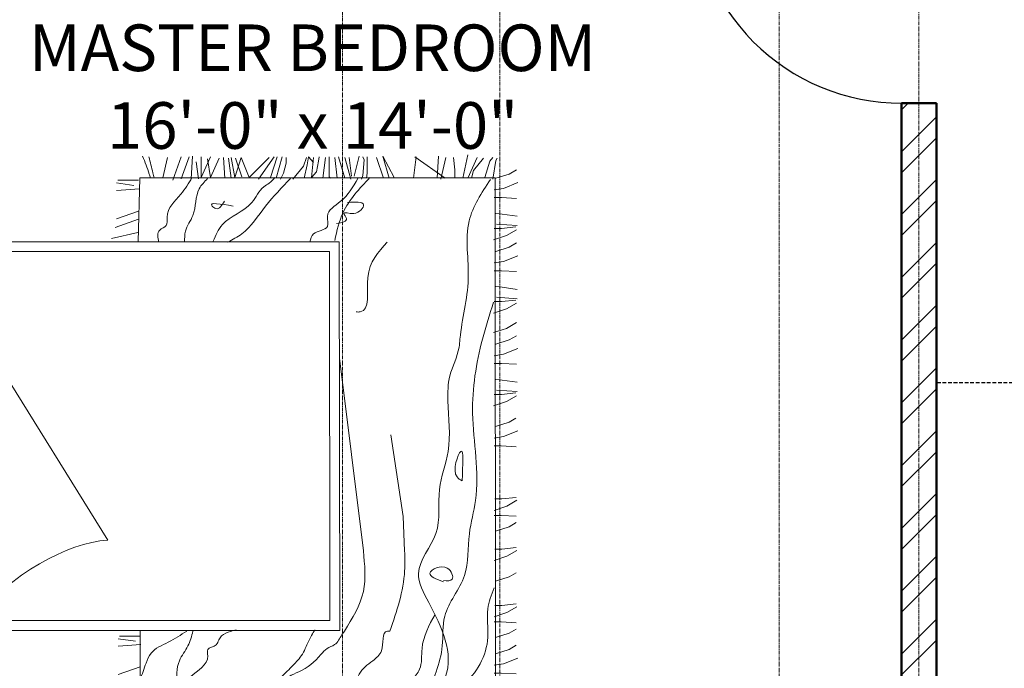
# Model space of a CAD drawing. Units: inches. Extents: x 261 to 2725, y 291 to 1454.
# Tile 5 of 35: x 519 to 688, y 549 to 661. Entities that reach past the tile are written whole.
import ezdxf

# ---------------------------------------------------------------- set-up
doc = ezdxf.new("R2010")
doc.units = ezdxf.units.IN
doc.linetypes.add('CENTER', pattern=[2, 1.25, -0.25, 0.25, -0.25])
doc.linetypes.add('DASHED', pattern=[19.05, 12.7, -6.35])
for name, color, linetype, lineweight in [('A-ANNO-DIMS', 136, 'Continuous', 18), ('A-AREA-IDEN', 18, 'Continuous', 18), ('A-DOOR', 160, 'Continuous', 25), ('A-FURN', 30, 'Continuous', 18), ('A-GRID', 251, 'CENTER', 13), ('A-WALL', 222, 'Continuous', 50), ('A-WALL-OVHD', 222, 'DASHED', 25), ('A-WALL-PATT', 243, 'Continuous', 13)]:
    doc.layers.add(name, color=color, linetype=linetype, lineweight=lineweight)
doc.styles.get("Standard").update_dxf_attribs({"font": 'arial.ttf'})
doc.dimstyles.new('ISO-25', dxfattribs={"dimtxt": 12, "dimasz": 6, "dimexe": 1.25, "dimexo": 0.625, "dimtad": 1, "dimdec": 0, "dimlunit": 3, "dimtxsty": 'Standard', "dimblk": 'ARCHTICK', "dimcen": 2.5, "dimadec": 0, "dimazin": 0, "dimtfac": 1, "dimtdec": 0, "dimtmove": 0, "dimatfit": 3, "dimfxl": 1, "dimfxlon": 1, "dimarcsym": 0})

# ---------------------------------------------------------------- blocks, each defined once
blk = doc.blocks.new('*U5')
for p, q in [((0, 0), (0, -4)), ((-36, 0), (-36, -4))]:
    blk.add_line(p, q)
blk.add_lwpolyline([(0, 0), (0, 36), (-1.75, 36), (-1.75, 0)], close=True)
blk.add_arc((0, 0), 36, 90, 180)
blk = doc.blocks.new('A$C2B723114')
for p, q in [((0, 2.9047), (2.8274, 2.9047)), ((0, 2.8487), (0, 2.9047)), ((2.8274, 2.9047), (2.8274, 2.8487)), ((2.8274, 2.8487), (0, 2.8487)), ((0.1012, 2.4649), (0.1012, 2.849)), ((0.1396, 2.5033), (0.1396, 2.849)), ((0.4243, 2.8697), (0.4243, 2.4855)), ((0.6794, 0.7051), (0.6794, 2.8509)), ((0.7187, 0.7435), (0.7187, 2.8509)), ((2.1776, 2.8509), (2.1776, 0.7454)), ((2.216, 2.8509), (2.216, 0.707)), ((2.4742, 2.8697), (2.4742, 2.4855)), ((2.6798, 2.5052), (2.6798, 2.8509)), ((2.7182, 2.4668), (2.7182, 2.8509)), ((0.6087, 2.6776), (0.295, 2.6776)), ((2.6586, 2.6776), (2.2821, 2.6776)), ((1.3789, 2.4999), (1.3598, 2.5761)), ((2.0593, 2.4999), (2.0402, 2.5761)), ((0.6766, 2.5033), (0.1396, 2.5033)), ((1.3858, 2.4723), (1.3789, 2.4999)), ((2.0662, 2.4723), (2.0593, 2.4999)), ((2.2188, 2.5052), (2.6798, 2.5052)), ((0.6794, 2.4649), (0.1012, 2.4649)), ((0.7191, 2.47), (2.1778, 2.4719)), ((2.2188, 2.4668), (2.7182, 2.4668)), ((2.1771, 2.3036), (0.718, 2.1685)), ((1.0365, 1.6233), (2.1246, 2.2989)), ((2.2287, 1.6076), (2.2523, 1.5035)), ((0.5047, 1.5819), (0.5353, 1.4945)), ((0.6174, 1.5819), (0.6232, 1.4916)), ((0.6467, 1.5819), (0.6369, 1.5137)), ((0.6571, 1.4945), (0.6571, 1.5765)), ((2.2726, 1.593), (2.3061, 1.5007)), ((2.3067, 1.5881), (2.3373, 1.5007)), ((2.4194, 1.5881), (2.4251, 1.4979)), ((2.4487, 1.5881), (2.4389, 1.5199)), ((2.4591, 1.5007), (2.4591, 1.5828)), ((0.4269, 0.0884), (0.4269, 1.4945)), ((0.4269, 1.4945), (0.6794, 1.4945)), ((2.4685, 1.4964), (2.216, 1.5022)), ((2.4685, 1.4964), (2.4685, 0.0903)), ((2.4685, 1.4044), (2.5491, 1.3861)), ((0.3172, 1.3923), (0.4213, 1.3687)), ((2.4596, 1.3659), (2.552, 1.3324)), ((0.3318, 1.3485), (0.4241, 1.3149)), ((2.4645, 1.3318), (2.552, 1.3012)), ((0.3367, 1.3143), (0.4241, 1.2838)), ((2.4645, 1.2928), (2.5548, 1.2871)), ((2.4645, 1.2635), (2.5328, 1.2733)), ((2.4699, 1.2531), (2.552, 1.2163)), ((2.552, 1.2531), (2.4699, 1.2531)), ((2.5435, 1.2276), (2.4699, 1.2163)), ((2.4699, 1.2163), (2.5463, 1.1823)), ((0.3367, 1.2016), (0.427, 1.1959)), ((0.3367, 1.1724), (0.405, 1.1821)), ((0.4241, 1.162), (0.3421, 1.162)), ((0.3421, 1.162), (0.4241, 1.1252)), ((2.5491, 1.1654), (2.467, 1.1597)), ((2.5463, 1.1455), (2.467, 1.1342)), ((2.5491, 1.1342), (2.4699, 1.1201)), ((2.4699, 1.1201), (2.5491, 1.0946)), ((2.5491, 1.0946), (2.4699, 1.0635)), ((2.5463, 1.1172), (2.4727, 1.0918)), ((2.4699, 1.0635), (2.5491, 0.9842)), ((0.4157, 1.0206), (0.3421, 1.0093)), ((2.4642, 1.0267), (2.552, 0.9644)), ((0.3421, 1.0093), (0.4185, 0.9754)), ((2.4699, 0.9785), (2.552, 0.9531)), ((0.4213, 0.9584), (0.3392, 0.9527)), ((0.4185, 0.9386), (0.3392, 0.9272)), ((2.4642, 0.9389), (2.4869, 0.9276)), ((2.467, 0.9559), (2.552, 0.9333)), ((0.4213, 0.9272), (0.3421, 0.9131)), ((0.3421, 0.9131), (0.4213, 0.8876)), ((0.4185, 0.9103), (0.3449, 0.8848)), ((2.4869, 0.9276), (2.5265, 0.9163)), ((2.5265, 0.9163), (2.5491, 0.9163)), ((0.4213, 0.8876), (0.3421, 0.8565)), ((2.4642, 0.8908), (2.5152, 0.8483)), ((0.3364, 0.8197), (0.4241, 0.7574)), ((0.3421, 0.8565), (0.4213, 0.7772)), ((2.467, 0.8455), (2.5208, 0.8342)), ((2.5152, 0.8483), (2.5491, 0.837)), ((2.5208, 0.8342), (2.552, 0.8285)), ((2.552, 0.8285), (2.5293, 0.8087)), ((2.4699, 0.8172), (2.4925, 0.7974)), ((2.5491, 0.8087), (2.4699, 0.8172)), ((2.4925, 0.7974), (2.535, 0.7889)), ((2.535, 0.7889), (2.552, 0.7861)), ((0.3392, 0.7489), (0.4241, 0.7263)), ((0.3421, 0.7716), (0.4241, 0.7461)), ((2.1776, 0.7454), (0.7187, 0.7435)), ((2.5491, 0.7606), (2.467, 0.7719)), ((2.4727, 0.7464), (2.467, 0.7408)), ((2.552, 0.7464), (2.4727, 0.7464)), ((0.359, 0.7206), (0.3987, 0.7093)), ((0.3987, 0.7093), (0.4213, 0.7093)), ((2.216, 0.707), (0.6794, 0.7051)), ((0.9938, 0.6115), (1.7555, 0.7064)), ((2.467, 0.7153), (2.5491, 0.7238)), ((2.552, 0.7096), (2.467, 0.6842)), ((2.5491, 0.6842), (2.4642, 0.6615)), ((2.5491, 0.6672), (2.4755, 0.6587)), ((0.3421, 0.6601), (0.4213, 0.5808)), ((2.4755, 0.6474), (2.5548, 0.6276)), ((0.3364, 0.6233), (0.4241, 0.561)), ((2.4642, 0.6191), (2.4784, 0.6134)), ((2.467, 0.5993), (2.4869, 0.5964)), ((2.4784, 0.6134), (2.5406, 0.6077)), ((2.4869, 0.5964), (2.552, 0.5964)), ((2.5406, 0.6077), (2.552, 0.6134)), ((0.3392, 0.5525), (0.4241, 0.5299)), ((0.3421, 0.5752), (0.4241, 0.5497)), ((2.467, 0.5313), (2.5491, 0.5596)), ((0.359, 0.5242), (0.3987, 0.5129)), ((2.467, 0.5087), (2.5548, 0.5342)), ((2.5548, 0.5342), (2.4699, 0.4889)), ((0.3364, 0.4785), (0.3874, 0.436)), ((1.4523, 0.5021), (1.1305, 0.4537)), ((0.3392, 0.4332), (0.393, 0.4219)), ((0.3874, 0.436), (0.4213, 0.4247)), ((1.1305, 0.4537), (0.9938, 0.448)), ((0.4213, 0.415), (0.3364, 0.3923)), ((0.4241, 0.2868), (0.3392, 0.415)), ((0.3421, 0.4049), (0.3647, 0.3851)), ((0.4213, 0.3964), (0.3421, 0.4049)), ((0.4213, 0.398), (0.3477, 0.3895)), ((0.393, 0.4219), (0.4241, 0.4162)), ((0.4241, 0.4162), (0.4015, 0.3964)), ((2.467, 0.4133), (2.552, 0.4019)), ((2.467, 0.2879), (2.552, 0.4076)), ((0.3647, 0.3851), (0.4072, 0.3766)), ((0.4072, 0.3766), (0.4241, 0.3738)), ((0.4213, 0.3377), (0.3392, 0.3491)), ((0.4241, 0.3236), (0.3449, 0.3236)), ((2.467, 0.319), (2.5548, 0.3134)), ((0.3392, 0.2925), (0.4213, 0.3009)), ((2.4642, 0.3049), (2.5491, 0.2851)), ((0.3477, 0.2571), (0.427, 0.2373)), ((2.4699, 0.2491), (2.501, 0.2491)), ((2.501, 0.2491), (2.5491, 0.2547)), ((0.3506, 0.2231), (0.4128, 0.2175)), ((0.359, 0.2061), (0.4241, 0.2061)), ((0.4128, 0.2175), (0.4241, 0.2231)), ((2.467, 0.2179), (2.5605, 0.1981)), ((2.467, 0.1981), (2.5491, 0.1613)), ((2.467, 0.184), (2.4982, 0.1755)), ((2.4982, 0.1755), (2.5463, 0.1359)), ((0.3392, 0.1042), (0.4213, 0.1325)), ((2.4699, 0.1302), (2.535, 0.1104)), ((0.3392, 0.0815), (0.427, 0.107)), ((0.427, 0.107), (0.3421, 0.0617)), ((2.4685, 0.0903), (0.4269, 0.0884)), ((0.5106, 0.094), (0.5106, 0.0657)), ((0.5417, 0.094), (0.5474, 0.0572)), ((0.587, 0.0884), (0.604, 0.0346)), ((0.6512, 0.0884), (0.6682, 0.0346)), ((0.713, 0.094), (0.713, 0.0657)), ((0.7334, 0.0943), (0.7503, 0.0434)), ((0.7786, 0.0915), (0.7786, 0.0632)), ((0.8739, 0.0884), (0.8908, 0.0346)), ((0.956, 0.0943), (0.973, 0.0434)), ((1.0013, 0.0915), (1.0013, 0.0632)), ((1.072, 0.0884), (1.089, 0.0346)), ((1.1338, 0.094), (1.1338, 0.0657)), ((1.1542, 0.0943), (1.1712, 0.0434)), ((1.1995, 0.0915), (1.1995, 0.0632)), ((1.4088, 0.094), (1.4088, 0.0657)), ((1.44, 0.094), (1.4456, 0.0572)), ((1.4853, 0.0884), (1.5023, 0.0346)), ((1.5674, 0.0962), (1.5844, 0.0453)), ((1.6127, 0.0934), (1.6127, 0.0651)), ((1.6297, 0.0849), (1.624, 0.0028)), ((1.6721, 0.0877), (1.6693, 0.0623)), ((1.7344, 0.0934), (1.7344, 0.0651)), ((1.7655, 0.0934), (1.7712, 0.0566)), ((1.8108, 0.0877), (1.8278, 0.034)), ((1.8568, 0.0962), (1.8738, 0.0453)), ((1.9342, 0.0962), (1.9512, 0.0453)), ((1.9795, 0.0934), (1.9795, 0.0651)), ((1.9965, 0.0849), (1.9908, 0.0028)), ((2.039, 0.0877), (2.0361, 0.0623)), ((2.1012, 0.0934), (2.1012, 0.0651)), ((2.1324, 0.0934), (2.138, 0.0566)), ((2.1777, 0.0877), (2.1946, 0.034)), ((2.2236, 0.0962), (2.2406, 0.0453)), ((2.2689, 0.0934), (2.2689, 0.0651)), ((2.2859, 0.0849), (2.2802, 0.0028)), ((2.3284, 0.0877), (2.3255, 0.0623)), ((2.3906, 0.0934), (2.3906, 0.0651)), ((2.4218, 0.0934), (2.4274, 0.0566)), ((2.4642, 0.0991), (2.5378, 0.0877)), ((2.467, 0.0877), (2.484, 0.034)), ((2.535, 0.1104), (2.5491, 0.0991)), ((2.5378, 0.0877), (2.5463, 0.0821)), ((0.5106, 0.0657), (0.5077, 0.0063)), ((0.5474, 0.0572), (0.57, 0.0006)), ((0.713, 0.0657), (0.7101, 0.0063)), ((0.7503, 0.0434), (0.773, 0.0037)), ((0.7786, 0.0632), (0.7843, 0.0066)), ((0.973, 0.0434), (0.9957, 0.0037)), ((1.0013, 0.0632), (1.007, 0.0066)), ((1.1338, 0.0657), (1.131, 0.0063)), ((1.1712, 0.0434), (1.1939, 0.0037)), ((1.1995, 0.0632), (1.2052, 0.0066)), ((1.4088, 0.0657), (1.406, 0.0063)), ((1.4456, 0.0572), (1.4683, 0.0006)), ((1.5844, 0.0453), (1.607, 0.0057)), ((1.6127, 0.0651), (1.6184, 0.0085)), ((1.6693, 0.0623), (1.6608, 0.0028)), ((1.7344, 0.0651), (1.7316, 0.0057)), ((1.7712, 0.0566), (1.7938, 0)), ((1.8738, 0.0453), (1.8964, 0.0057)), ((1.9512, 0.0453), (1.9739, 0.0057)), ((1.9795, 0.0651), (1.9852, 0.0085)), ((2.0361, 0.0623), (2.0276, 0.0028)), ((2.1012, 0.0651), (2.0984, 0.0057)), ((2.138, 0.0566), (2.1607, 0)), ((2.2406, 0.0453), (2.2632, 0.0057)), ((2.2689, 0.0651), (2.2746, 0.0085)), ((2.3255, 0.0623), (2.317, 0.0028)), ((2.3906, 0.0651), (2.3878, 0.0057)), ((2.4274, 0.0566), (2.4501, 0)), ((0.604, 0.0346), (0.621, 0.0063)), ((0.6682, 0.0346), (0.6851, 0.0063)), ((0.8908, 0.0346), (0.9078, 0.0063)), ((1.089, 0.0346), (1.106, 0.0063)), ((1.5023, 0.0346), (1.5192, 0.0082)), ((1.8278, 0.034), (1.8448, 0.0057)), ((2.1946, 0.034), (2.2116, 0.0057)), ((2.484, 0.034), (2.501, 0.0057))]:
    blk.add_line(p, q)
for centre, radius in [((0.4243, 2.6776), 0.0821), ((2.4742, 2.6776), 0.0821), ((0.4243, 2.6776), 0.0493), ((2.4742, 2.6776), 0.0493)]:
    blk.add_circle(centre, radius)
for centre, radius, start, end in [((0.8078, 2.821), 0.00214, 160.436, 281.8931), ((0.8088, 2.8207), 0.00315, 111.7883, 160.436), ((0.8162, 2.8021), 0.0232, 94.3025, 111.7883), ((0.8091, 2.8151), 0.00394, 21.9904, 101.8931), ((0.8409, 2.7949), 0.0302, 158.579, 188.1335), ((0.7994, 2.8112), 0.0144, 338.579, 21.9904), ((0.8165, 2.7987), 0.0266, 59.3487, 94.3025), ((0.8554, 2.8643), 0.0497, 239.3487, 264.7408), ((0.9202, 3.5684), 0.7568, 264.7408, 268.0921), ((0.8679, 2.7254), 0.0915, 74.0648, 94.2159), ((0.8679, 2.7254), 0.0915, 53.9136, 74.0648), ((0.9409, 4.189), 1.3777, 268.0921, 270.5757), ((0.86, 2.6097), 0.2158, 62.7604, 69.1397), ((0.9466, 3.6164), 0.8051, 270.5757, 274.8018), ((1.0364, 2.548), 0.2671, 87.4614, 94.8018), ((1.042, 2.6745), 0.1405, 79.8101, 87.4614), ((1.1532, 3.2931), 0.488, 259.8101, 263.9133), ((1.204, 3.7695), 0.9671, 263.9133, 270), ((1.204, 3.4318), 0.6294, 270, 277.5469), ((1.2573, 3.0292), 0.2233, 277.5469, 285.744), ((1.3941, 2.5438), 0.281, 98.4372, 105.744), ((1.3747, 2.6748), 0.1486, 90, 98.4372), ((1.3747, 2.74), 0.0833, 78.7276, 90), ((1.3886, 2.8099), 0.0121, 333.4195, 78.7276), ((1.4882, 2.821), 0.00214, 160.436, 281.8931), ((1.4892, 2.8207), 0.00315, 111.7883, 160.436), ((1.4966, 2.8021), 0.0232, 94.3025, 111.7883), ((1.4895, 2.8151), 0.00394, 21.9904, 101.8931), ((1.5213, 2.7949), 0.0302, 158.579, 188.1335), ((1.4798, 2.8112), 0.0144, 338.579, 21.9904), ((1.4969, 2.7987), 0.0266, 59.3487, 94.3025), ((1.5358, 2.8643), 0.0497, 239.3487, 264.7408), ((1.6006, 3.5684), 0.7568, 264.7408, 268.0921), ((1.5483, 2.7254), 0.0915, 74.0648, 94.2159), ((1.5483, 2.7254), 0.0915, 53.9136, 74.0648), ((1.6213, 4.189), 1.3777, 268.0921, 270.5757), ((1.5404, 2.6097), 0.2158, 62.7604, 69.1397), ((1.627, 3.6164), 0.8051, 270.5757, 274.8018), ((1.7168, 2.548), 0.2671, 87.4614, 94.8018), ((1.7224, 2.6745), 0.1405, 79.8101, 87.4614), ((1.8336, 3.2931), 0.488, 259.8101, 263.9133), ((1.8844, 3.7695), 0.9671, 263.9133, 270), ((1.8844, 3.4318), 0.6294, 270, 277.5469), ((1.9377, 3.0292), 0.2233, 277.5469, 285.744), ((2.0745, 2.5438), 0.281, 98.4372, 105.744), ((2.0551, 2.6748), 0.1486, 90, 98.4372), ((2.0551, 2.74), 0.0833, 78.7276, 90), ((2.069, 2.8099), 0.0121, 333.4195, 78.7276), ((1.0356, 2.8227), 0.2268, 188.1335, 192.1095), ((0.635, 2.7368), 0.1829, 7.6809, 12.1095), ((0.8679, 2.7254), 0.0915, 36.1766, 53.9136), ((0.8679, 2.7254), 0.0915, 18.4397, 36.1766), ((0.9263, 2.7386), 0.0708, 51.6114, 62.7604), ((0.7461, 2.511), 0.3611, 46.1885, 51.6114), ((0.8523, 2.6218), 0.2076, 39.0349, 46.1885), ((1.3713, 2.8186), 0.0315, 274.4002, 333.4195), ((0.923, 2.7382), 0.4535, 0, 6.2324), ((1.716, 2.8227), 0.2268, 188.1335, 192.1095), ((1.3154, 2.7368), 0.1829, 7.6809, 12.1095), ((1.5483, 2.7254), 0.0915, 36.1766, 53.9136), ((1.5483, 2.7254), 0.0915, 18.4397, 36.1766), ((1.6067, 2.7386), 0.0708, 51.6114, 62.7604), ((1.4265, 2.511), 0.3611, 46.1885, 51.6114), ((1.5327, 2.6218), 0.2076, 39.0349, 46.1885), ((2.0517, 2.8186), 0.0315, 274.4002, 333.4195), ((1.6034, 2.7382), 0.4535, 0, 6.2324), ((-0.0181, 2.6487), 0.8418, 3.3687, 7.6809), ((0.9783, 2.7239), 0.0455, 28.3168, 39.0349), ((0.8558, 2.6579), 0.1846, 23.0028, 28.3168), ((1.1884, 2.7382), 0.1881, 350.3156, 0), ((0.6623, 2.6487), 0.8418, 3.3687, 7.6809), ((1.6587, 2.7239), 0.0455, 28.3168, 39.0349), ((1.5362, 2.6579), 0.1846, 23.0028, 28.3168), ((1.8688, 2.7382), 0.1881, 350.3156, 0), ((0.1976, 2.6614), 0.6258, 358.3669, 3.3687), ((0.5722, 2.8434), 0.8132, 347.8016, 350.3156), ((0.878, 2.6614), 0.6258, 358.3669, 3.3687), ((1.2526, 2.8434), 0.8132, 347.8016, 350.3156), ((1.9648, 2.5659), 0.6074, 171.9949, 177.3351), ((1.6528, 2.6098), 0.2924, 167.8016, 171.9949), ((2.6452, 2.5659), 0.6074, 171.9949, 177.3351), ((2.3332, 2.6098), 0.2924, 167.8016, 171.9949), ((-11.7321, 3.2823), 12.5718, 356.49514, 356.94504), ((-0.4351, 2.6794), 1.2587, 356.945, 358.3669), ((-11.0517, 3.2823), 12.5718, 356.49514, 356.94504), ((0.2453, 2.6794), 1.2587, 356.945, 358.3669), ((1.4204, 2.5912), 0.0624, 177.3351, 194.0452), ((2.1008, 2.5912), 0.0624, 177.3351, 194.0452), ((0.5206, 2.5319), 0.2961, 350.0016, 356.4951), ((1.4917, 3.1364), 0.681, 244.6889, 246.5156), ((1.4917, 3.1364), 0.681, 246.5156, 248.3423), ((1.4917, 3.1364), 0.681, 248.3423, 250.572), ((1.4917, 3.1364), 0.681, 250.572, 252.8018), ((1.201, 2.5319), 0.2961, 350.0016, 356.4951), ((2.1721, 3.1364), 0.681, 244.6889, 246.5156), ((2.1721, 3.1364), 0.681, 246.5156, 248.3423), ((2.1721, 3.1364), 0.681, 248.3423, 250.572), ((2.1721, 3.1364), 0.681, 250.572, 252.8018), ((0.8298, 2.4774), 0.0178, 170.0016, 196.6978), ((0.8139, 2.4726), 0.00122, 196.6978, 277.1204), ((0.8041, 2.5514), 0.0807, 277.1204, 286.2212), ((0.8068, 2.5419), 0.0707, 286.2212, 297.2841), ((0.8584, 2.4419), 0.0418, 102.869, 117.2841), ((0.879, 2.3515), 0.1345, 93.574, 102.869), ((0.9376, 1.4146), 1.0732, 90.2865, 93.574), ((0.9586, -2.7845), 5.2724, 89.0296, 90.2865), ((0.9954, -0.6123), 3.0999, 87.3904, 89.0296), ((1.0854, 1.364), 1.1216, 85.3824, 87.3904), ((1.28, 3.7729), 1.2952, 265.3824, 267.2509), ((1.228, 2.691), 0.2121, 267.2509, 281.5586), ((1.2975, 2.3514), 0.1345, 83.5659, 101.5586), ((1.3002, 2.3754), 0.1104, 72.6136, 83.5659), ((1.3965, 2.6828), 0.2118, 252.6136, 260.5159), ((1.4027, 2.7202), 0.2496, 260.5159, 265.9171), ((1.385, 2.4721), 0.000845, 265.9171, 14.0449), ((1.5102, 2.4774), 0.0178, 170.0016, 196.6978), ((1.4943, 2.4726), 0.00122, 196.6978, 277.1204), ((1.4845, 2.5514), 0.0807, 277.1204, 286.2212), ((1.4872, 2.5419), 0.0707, 286.2212, 297.2841), ((1.5388, 2.4419), 0.0418, 102.869, 117.2841), ((1.5594, 2.3515), 0.1345, 93.574, 102.869), ((1.618, 1.4146), 1.0732, 90.2865, 93.574), ((1.639, -2.7845), 5.2724, 89.0296, 90.2865), ((1.6758, -0.6123), 3.0999, 87.3904, 89.0296), ((1.7658, 1.364), 1.1216, 85.3824, 87.3904), ((1.9604, 3.7729), 1.2952, 265.3824, 267.2509), ((1.9084, 2.691), 0.2121, 267.2509, 281.5586), ((1.9779, 2.3514), 0.1345, 83.5659, 101.5586), ((1.9806, 2.3754), 0.1104, 72.6136, 83.5659), ((2.0769, 2.6828), 0.2118, 252.6136, 260.5159), ((2.0831, 2.7202), 0.2496, 260.5159, 265.9171), ((2.0654, 2.4721), 0.000845, 265.9171, 14.0449)]:
    blk.add_arc(centre, radius, start, end)
blk.add_ellipse((0.4962, 1.9132), major_axis=(0.4887, -0.4605), ratio=0.503305, start_param=0.491272, end_param=1.591113)
for points, knots in [([(0.6768, 1.3104), (0.6615, 1.3339), (0.6315, 1.3797), (0.604, 1.4501), (0.5417, 1.4748), (0.5064, 1.4871), (0.4848, 1.4945)], [0, 0, 0, 0, 110.980521, 216.571322, 273.316778, 363.252298, 363.252298, 363.252298, 363.252298]), ([(2.5548, 1.4853), (2.5314, 1.4757), (2.5031, 1.4641), (2.4737, 1.4555), (2.4685, 1.454)], [0, 0, 0, 0, 98.452083, 119.481049, 119.481049, 119.481049, 119.481049]), ([(0.427, 1.4678), (0.4036, 1.4582), (0.3693, 1.4441), (0.3335, 1.4344), (0.3221, 1.4313)], [0, 0, 0, 0, 98.452083, 144.639601, 144.639601, 144.639601, 144.639601]), ([(0.4241, 1.4423), (0.4031, 1.437), (0.3691, 1.4284), (0.3351, 1.4199), (0.3221, 1.4167)], [0, 0, 0, 0, 84.638756, 136.955563, 136.955563, 136.955563, 136.955563]), ([(2.552, 1.4598), (2.5309, 1.4545), (2.5031, 1.4475), (2.4753, 1.4406), (2.4685, 1.4389)], [0, 0, 0, 0, 84.638756, 111.94623, 111.94623, 111.94623, 111.94623]), ([(2.2145, 1.4211), (2.233, 1.4246), (2.2636, 1.4303), (2.2761, 1.3837), (2.3429, 1.3967), (2.3949, 1.3342), (2.4474, 1.3031), (2.4698, 1.2898)], [0, 0, 0, 0, 61.886907, 102.717887, 145.699352, 284.082577, 386.765171, 386.765171, 386.765171, 386.765171]), ([(0.6768, 1.286), (0.6567, 1.2911), (0.6145, 1.3017), (0.5543, 1.3533), (0.4816, 1.349), (0.4362, 1.3493), (0.4233, 1.3493)], [0, 0, 0, 0, 80.250278, 168.388677, 295.908361, 346.663112, 346.663112, 346.663112, 346.663112]), ([(0.4233, 1.3445), (0.4367, 1.3385), (0.464, 1.3264), (0.5129, 1.2848), (0.5456, 1.2161), (0.6131, 1.2349), (0.6142, 1.1913), (0.6642, 1.1806), (0.674, 1.144), (0.6817, 1.1154)], [0, 0, 0, 0, 56.745495, 115.23739, 254.956954, 286.678662, 337.828324, 366.201072, 468.500395, 468.500395, 468.500395, 468.500395]), ([(2.2145, 1.319), (2.2295, 1.319), (2.2678, 1.3192), (2.3288, 1.2705), (2.4143, 1.279), (2.4535, 1.2403), (2.4662, 1.2278)], [0, 0, 0, 0, 57.155505, 146.33427, 287.936209, 355.396728, 355.396728, 355.396728, 355.396728]), ([(2.3573, 1.127), (2.3656, 1.1759), (2.3758, 1.2352), (2.3371, 1.1853), (2.3602, 1.1713), (2.3768, 1.1612)], [0, 0, 0, 0, 107.853607, 130.728419, 189.220329, 189.220329, 189.220329, 189.220329]), ([(2.2182, 1.2059), (2.2419, 1.1958), (2.3116, 1.1659), (2.342, 1.0552), (2.4266, 1.0223), (2.4474, 0.9811), (2.462, 0.9684), (2.4698, 0.9616)], [0, 0, 0, 0, 97.73655, 287.59661, 389.176293, 423.403759, 463.679181, 463.679181, 463.679181, 463.679181]), ([(2.2145, 1.1476), (2.2246, 1.1286), (2.2575, 1.0666), (2.3612, 1.0009), (2.431, 0.9336), (2.4662, 0.8996)], [0, 0, 0, 0, 83.02987, 271.460712, 463.033803, 463.033803, 463.033803, 463.033803]), ([(0.6817, 0.8034), (0.6673, 0.8119), (0.6341, 0.8315), (0.5785, 0.8518), (0.5349, 0.8973), (0.4828, 0.9461), (0.4518, 0.9879), (0.4331, 1.013)], [0, 0, 0, 0, 65.318952, 150.437229, 226.833166, 307.58338, 429.454095, 429.454095, 429.454095, 429.454095]), ([(0.4282, 0.9448), (0.4547, 0.9353), (0.496, 0.9206), (0.5223, 0.8436), (0.5628, 0.7946), (0.6113, 0.7575), (0.6214, 0.7173), (0.6539, 0.7022), (0.672, 0.6897), (0.6768, 0.6864)], [0, 0, 0, 0, 102.299436, 159.044876, 303.717955, 348.579152, 391.138254, 454.581655, 477.456496, 477.456496, 477.456496, 477.456496]), ([(2.2145, 0.823), (2.227, 0.8201), (2.261, 0.8121), (2.261, 0.7401), (2.3352, 0.7659), (2.379, 0.6836), (2.4336, 0.6521), (2.4662, 0.6334)], [0, 0, 0, 0, 46.747668, 127.438174, 179.649794, 280.561838, 429.605131, 429.605131, 429.605131, 429.605131]), ([(0.4282, 0.74), (0.4347, 0.7029), (0.444, 0.6496), (0.5194, 0.6274), (0.555, 0.5807), (0.5975, 0.5243), (0.6789, 0.5415), (0.677, 0.5095), (0.6768, 0.5061)], [0, 0, 0, 0, 130.791737, 187.537266, 286.231946, 353.673191, 460.023761, 472.712403, 472.712403, 472.712403, 472.712403]), ([(2.2218, 0.7246), (2.2595, 0.716), (2.3548, 0.6945), (2.4265, 0.6268), (2.4698, 0.586)], [0, 0, 0, 0, 148.665024, 375.555892, 375.555892, 375.555892, 375.555892]), ([(2.3719, 0.6737), (2.3738, 0.6431), (2.3772, 0.5878), (2.3146, 0.6382), (2.3401, 0.7015), (2.2971, 0.6649), (2.2923, 0.6965), (2.289, 0.7176)], [0, 0, 0, 0, 83.446591, 150.887818, 201.642461, 230.015204, 286.760644, 286.760644, 286.760644, 286.760644]), ([(0.6768, 0.6864), (0.7275, 0.655), (0.8251, 0.5944), (0.9391, 0.606), (0.9938, 0.6115)], [0, 0, 0, 0, 225.995823, 434.686543, 434.686543, 434.686543, 434.686543]), ([(2.2145, 0.5167), (2.1764, 0.5522), (2.1051, 0.6184), (1.9357, 0.5803), (1.9385, 0.6342), (1.9388, 0.6395)], [0, 0, 0, 0, 208.073343, 389.01094, 409.01094, 409.01094, 409.01094, 409.01094]), ([(0.6768, 0.5061), (0.7554, 0.4794), (0.8591, 0.4442), (0.9675, 0.4473), (0.9938, 0.448)], [0, 0, 0, 0, 319.374611, 421.61723, 421.61723, 421.61723, 421.61723]), ([(0.4331, 0.4427), (0.4498, 0.4356), (0.4827, 0.4216), (0.5314, 0.3759), (0.632, 0.3884), (0.6996, 0.3513), (0.7423, 0.3278)], [0, 0, 0, 0, 70.931849, 139.556414, 248.154027, 434.709995, 434.709995, 434.709995, 434.709995]), ([(2.4625, 0.1088), (2.4095, 0.1438), (2.2904, 0.2226), (2.0623, 0.1771), (1.9006, 0.2246), (1.7699, 0.2337), (1.6941, 0.2766), (1.5528, 0.2786), (1.4005, 0.2587), (1.2324, 0.3267), (1.059, 0.2939), (0.9218, 0.426), (0.7359, 0.3204), (0.5586, 0.2391), (0.4502, 0.3116), (0.427, 0.3272)], [0, 0, 0, 0, 239.874704, 538.942419, 850.40885, 893.390315, 1047.998294, 1176.505142, 1437.500972, 1637.333004, 1864.324391, 2089.058767, 2248.736533, 2637.953392, 2744.252142, 2744.252142, 2744.252142, 2744.252142]), ([(1.9771, 0.0962), (1.9286, 0.1117), (1.7864, 0.157), (1.5223, 0.1992), (1.2611, 0.141), (1.0527, 0.2023), (0.8859, 0.1885), (0.76, 0.3042), (0.6211, 0.292), (0.5187, 0.3203), (0.4572, 0.3456), (0.4282, 0.3575)], [0, 0, 0, 0, 198.710624, 582.73994, 1031.873213, 1206.082894, 1423.278209, 1655.952104, 1808.744089, 1945.69963, 2068.229211, 2068.229211, 2068.229211, 2068.229211]), ([(0.8474, 0.0943), (0.82, 0.1047), (0.757, 0.1287), (0.6201, 0.1029), (0.4623, 0.1837), (0.4372, 0.2936), (0.4282, 0.3331)], [0, 0, 0, 0, 112.422038, 258.341957, 533.791494, 688.286079, 688.286079, 688.286079, 688.286079]), ([(0.8718, 0.2941), (0.8821, 0.3221), (0.9041, 0.3814), (0.9523, 0.2773), (0.8733, 0.2454), (0.8757, 0.2798), (0.8766, 0.2941)], [0, 0, 0, 0, 82.720021, 175.094899, 237.579423, 282.440623, 282.440623, 282.440623, 282.440623]), ([(1.2715, 0.221), (1.3344, 0.2172), (1.4529, 0.21), (1.2971, 0.2665), (1.2756, 0.2284), (1.2715, 0.221)], [0, 0, 0, 0, 150.888188, 283.977876, 315.699589, 315.699589, 315.699589, 315.699589])]:
    blk.add_open_spline(points, degree=3, knots=knots)
blk = doc.blocks.new('_ArchTick')
at = {"color": 0, "linetype": 'ByBlock', "const_width": 0.15}
blk.add_lwpolyline([(-0.5, -0.5), (0.5, 0.5)], dxfattribs=at)
blk = doc.blocks.new('*D86')
at = {"layer": 'A-ANNO-DIMS', "color": 0, "lineweight": -2, "ltscale": 0.07, "transparency": 16777216}
for p, q in [((676.45, 1437.76), (676.45, 1440.01)), ((772.45, 1437.76), (772.45, 1440.01)), ((676.45, 1438.76), (772.45, 1438.76))]:
    blk.add_line(p, q, dxfattribs=at)
at = {"layer": 'Defpoints', "color": 0, "ltscale": 0.07, "transparency": 16777216}
for p in [(772.45, 1438.76), (676.45, 517.47), (772.45, 517.47)]:
    blk.add_point(p, dxfattribs=at)
at = {"layer": 'A-ANNO-DIMS', "color": 0, "lineweight": -2, "ltscale": 0.07, "transparency": 16777216, "xscale": 6, "yscale": 6, "zscale": 6, "rotation": 180}
blk.add_blockref('_ArchTick', (676.45, 1438.76), dxfattribs=at)
at = {"layer": 'A-ANNO-DIMS', "color": 0, "lineweight": -2, "ltscale": 0.07, "transparency": 16777216, "xscale": 6, "yscale": 6, "zscale": 6}
blk.add_blockref('_ArchTick', (772.45, 1438.76), dxfattribs=at)
at = {"layer": 'A-ANNO-DIMS', "color": 0, "ltscale": 0.07, "transparency": 16777216, "insert": (724.45, 1445.51), "char_height": 12, "attachment_point": 5}
blk.add_mtext('8\'-0"', dxfattribs=at)
blk = doc.blocks.new('*D96')
at = {"layer": 'A-ANNO-DIMS', "color": 0, "lineweight": -2, "ltscale": 0.07, "transparency": 16777216}
for p, q in [((577.45, 305.22), (577.45, 302.97)), ((670.45, 305.22), (670.45, 302.97)), ((577.45, 304.22), (670.45, 304.22))]:
    blk.add_line(p, q, dxfattribs=at)
at = {"layer": 'Defpoints', "color": 0, "ltscale": 0.07, "transparency": 16777216}
for p in [(577.45, 775.47), (670.45, 775.47), (670.45, 304.22)]:
    blk.add_point(p, dxfattribs=at)
at = {"layer": 'A-ANNO-DIMS', "color": 0, "lineweight": -2, "ltscale": 0.07, "transparency": 16777216, "xscale": 6, "yscale": 6, "zscale": 6, "rotation": 180}
blk.add_blockref('_ArchTick', (577.45, 304.22), dxfattribs=at)
at = {"layer": 'A-ANNO-DIMS', "color": 0, "lineweight": -2, "ltscale": 0.07, "transparency": 16777216, "xscale": 6, "yscale": 6, "zscale": 6}
blk.add_blockref('_ArchTick', (670.45, 304.22), dxfattribs=at)
at = {"layer": 'A-ANNO-DIMS', "color": 0, "ltscale": 0.07, "transparency": 16777216, "insert": (623.95, 310.97), "char_height": 12, "attachment_point": 5}
blk.add_mtext('7\'-9"', dxfattribs=at)
blk = doc.blocks.new('*D98')
at = {"layer": 'A-ANNO-DIMS', "color": 0, "lineweight": -2, "ltscale": 0.07, "transparency": 16777216}
for p, q in [((287.06, 682.47), (284.81, 682.47)), ((286.06, 682.47), (286.06, 646.47)), ((287.06, 646.47), (284.81, 646.47))]:
    blk.add_line(p, q, dxfattribs=at)
at = {"layer": 'Defpoints', "color": 0, "ltscale": 0.07, "transparency": 16777216}
for p in [(676.45, 682.47), (286.06, 646.47), (676.45, 646.47)]:
    blk.add_point(p, dxfattribs=at)
at = {"layer": 'A-ANNO-DIMS', "color": 0, "lineweight": -2, "ltscale": 0.07, "transparency": 16777216, "xscale": 6, "yscale": 6, "zscale": 6}
for p, rotation in [((286.06, 682.47), 90), ((286.06, 646.47), 270)]:
    blk.add_blockref('_ArchTick', p, dxfattribs=dict(at, rotation=rotation))
at = {"layer": 'A-ANNO-DIMS', "color": 0, "ltscale": 0.07, "transparency": 16777216, "insert": (279.3, 664.47), "char_height": 12, "attachment_point": 5, "rotation": 90}
blk.add_mtext('3\'-0"', dxfattribs=at)
blk = doc.blocks.new('*D103')
at = {"layer": 'A-ANNO-DIMS', "color": 0, "lineweight": -2, "ltscale": 0.07, "transparency": 16777216}
for p, q in [((287.06, 1231.47), (284.81, 1231.47)), ((286.06, 439.47), (286.06, 1231.47)), ((287.06, 439.47), (284.81, 439.47))]:
    blk.add_line(p, q, dxfattribs=at)
at = {"layer": 'Defpoints', "color": 0, "ltscale": 0.07, "transparency": 16777216}
for p in [(286.06, 1231.47), (1243.08, 1231.47), (1243.08, 439.47)]:
    blk.add_point(p, dxfattribs=at)
at = {"layer": 'A-ANNO-DIMS', "color": 0, "lineweight": -2, "ltscale": 0.07, "transparency": 16777216, "xscale": 6, "yscale": 6, "zscale": 6}
for p, rotation in [((286.06, 1231.47), 90), ((286.06, 439.47), 270)]:
    blk.add_blockref('_ArchTick', p, dxfattribs=dict(at, rotation=rotation))
at = {"layer": 'A-ANNO-DIMS', "color": 0, "ltscale": 0.07, "transparency": 16777216, "insert": (279.3, 835.47), "char_height": 12, "attachment_point": 5, "rotation": 90}
blk.add_mtext('66\'-0"', dxfattribs=at)
blk = doc.blocks.new('*D107')
at = {"layer": 'A-ANNO-DIMS', "color": 0, "lineweight": -2, "ltscale": 0.07, "transparency": 16777216}
for p, q in [((287.06, 673.47), (284.81, 673.47)), ((286.06, 496.47), (286.06, 673.47)), ((287.06, 496.47), (284.81, 496.47))]:
    blk.add_line(p, q, dxfattribs=at)
at = {"layer": 'Defpoints', "color": 0, "ltscale": 0.07, "transparency": 16777216}
for p in [(286.06, 673.47), (1252.08, 673.47), (1252.08, 496.47)]:
    blk.add_point(p, dxfattribs=at)
at = {"layer": 'A-ANNO-DIMS', "color": 0, "lineweight": -2, "ltscale": 0.07, "transparency": 16777216, "xscale": 6, "yscale": 6, "zscale": 6}
for p, rotation in [((286.06, 673.47), 90), ((286.06, 496.47), 270)]:
    blk.add_blockref('_ArchTick', p, dxfattribs=dict(at, rotation=rotation))
at = {"layer": 'A-ANNO-DIMS', "color": 0, "ltscale": 0.07, "transparency": 16777216, "insert": (279.3, 584.97), "char_height": 12, "attachment_point": 5, "rotation": 90}
blk.add_mtext('14\'-9"', dxfattribs=at)
blk = doc.blocks.new('*D123')
at = {"layer": 'A-ANNO-DIMS', "color": 0, "lineweight": -2, "ltscale": 0.07, "transparency": 16777216}
for p, q in [((287.06, 1054.85), (284.81, 1054.85)), ((286.06, 439.47), (286.06, 1054.85)), ((287.06, 439.47), (284.81, 439.47))]:
    blk.add_line(p, q, dxfattribs=at)
at = {"layer": 'Defpoints', "color": 0, "ltscale": 0.07, "transparency": 16777216}
for p in [(286.06, 1054.85), (2007.71, 1054.85), (2007.71, 439.47)]:
    blk.add_point(p, dxfattribs=at)
at = {"layer": 'A-ANNO-DIMS', "color": 0, "lineweight": -2, "ltscale": 0.07, "transparency": 16777216, "xscale": 6, "yscale": 6, "zscale": 6}
for p, rotation in [((286.06, 1054.85), 90), ((286.06, 439.47), 270)]:
    blk.add_blockref('_ArchTick', p, dxfattribs=dict(at, rotation=rotation))
at = {"layer": 'A-ANNO-DIMS', "color": 0, "ltscale": 0.07, "transparency": 16777216, "insert": (279.22, 747.16), "char_height": 12, "attachment_point": 5, "rotation": 90}
blk.add_mtext('51\'-3 1/2"', dxfattribs=at)

msp = doc.modelspace()

# ---------------------------------------------------------------- hatches: boundary and pattern name
at = {"layer": 'A-WALL-PATT'}
h = msp.add_hatch(dxfattribs=at)
h.set_pattern_fill('ANSI32', color=256, scale=0.8)
h.paths.add_polyline_path([(478.45, 685.47), (580.45, 685.47), (580.45, 691.47), (577.45, 691.47), (577.45, 694.47), (571.45, 694.47), (571.45, 691.47), (478.45, 691.47), (478.45, 721.47), (469.45, 721.47), (469.45, 508.47), (538.45, 508.47), (538.45, 517.47), (478.45, 517.47)])
h.paths.add_polyline_path([(694.45, 517.47), (676.45, 517.47), (676.45, 646.47), (670.45, 646.47), (670.45, 517.47), (610.45, 517.47), (610.45, 508.47), (694.45, 508.47)])
h.paths.add_polyline_path([(676.45, 784.47), (478.45, 784.47), (478.45, 844.47), (469.45, 844.47), (469.45, 745.47), (478.45, 745.47), (478.45, 775.47), (571.45, 775.47), (571.45, 724.47), (577.45, 724.47), (577.45, 775.47), (670.45, 775.47), (670.45, 691.47), (610.45, 691.47), (610.45, 685.47), (670.45, 685.47), (670.45, 682.47), (676.45, 682.47)])
h.paths.add_polyline_path([(955.45, 880.47), (946.45, 880.47), (946.45, 808.47), (778.45, 808.47), (778.45, 799.47), (946.45, 799.47), (946.45, 517.47), (898.45, 517.47), (898.45, 508.47), (955.45, 508.47)])
h.paths.add_polyline_path([(778.45, 598.47), (772.45, 598.47), (772.45, 517.47), (754.45, 517.47), (754.45, 508.47), (826.45, 508.47), (826.45, 517.47), (778.45, 517.47)])
h.paths.add_polyline_path([(955.45, 1090.47), (946.45, 1090.47), (946.45, 1030.47), (817.45, 1030.47), (817.45, 1024.47), (946.45, 1024.47), (946.45, 952.47), (955.45, 952.47)])
h.paths.add_polyline_path([(955.45, 1231.47), (730.45, 1231.47), (730.45, 1222.47), (772.45, 1222.47), (772.45, 1096.47), (766.45, 1096.47), (766.45, 1090.47), (772.45, 1090.47), (772.45, 1006.47), (712.45, 1006.47), (712.45, 1000.47), (778.45, 1000.47), (778.45, 1024.47), (781.45, 1024.47), (781.45, 1030.47), (778.45, 1030.47), (778.45, 1222.47), (946.45, 1222.47), (946.45, 1162.47), (955.45, 1162.47)])
h.paths.add_polyline_path([(694.45, 1231.47), (619.45, 1231.47), (619.45, 1222.47), (646.45, 1222.47), (646.45, 1039.47), (652.45, 1039.47), (652.45, 1090.47), (736.45, 1090.47), (736.45, 1096.47), (652.45, 1096.47), (652.45, 1222.47), (694.45, 1222.47)])
h.paths.add_polyline_path([(571.45, 1231.47), (469.45, 1231.47), (469.45, 1099.47), (478.45, 1099.47), (478.45, 1144.47), (544.45, 1144.47), (544.45, 1153.47), (538.45, 1153.47), (538.45, 1150.47), (478.45, 1150.47), (478.45, 1222.47), (538.45, 1222.47), (538.45, 1183.47), (544.45, 1183.47), (544.45, 1222.47), (571.45, 1222.47)])
h.paths.add_polyline_path([(538.45, 1006.47), (478.45, 1006.47), (478.45, 1051.47), (469.45, 1051.47), (469.45, 940.47), (478.45, 940.47), (478.45, 1000.47), (538.45, 1000.47)])
h.paths.add_polyline_path([(652.45, 1006.47), (652.45, 1009.47), (646.45, 1009.47), (646.45, 1006.47), (586.45, 1006.47), (586.45, 1000.47), (652.45, 1000.47)])
h.paths.add_polyline_path([(1288.08, 973.47), (1243.08, 973.47), (1243.08, 920.97), (1252.08, 920.97), (1252.08, 964.47), (1288.08, 964.47)], flags=17)
h.paths.add_polyline_path([(1402.08, 805.47), (1252.08, 805.47), (1252.08, 848.97), (1243.08, 848.97), (1243.08, 757.47), (1252.08, 757.47), (1252.08, 799.47), (1294.08, 799.47), (1372.08, 799.47), (1372.08, 779.47), (1372.08, 715.47), (1378.08, 715.47), (1378.08, 799.47), (1402.08, 799.47)])
h.paths.add_polyline_path([(1252.08, 721.47), (1243.08, 721.47), (1243.08, 439.47), (1729.08, 439.47), (1729.08, 709.47), (1720.08, 709.47), (1720.08, 679.47), (1582.08, 679.47), (1582.08, 670.47), (1588.08, 670.47), (1588.08, 673.47), (1720.08, 673.47), (1720.08, 559.47), (1690.08, 559.47), (1690.08, 550.47), (1720.08, 550.47), (1720.08, 448.47), (1252.08, 448.47), (1252.08, 496.47), (1312.08, 496.47), (1312.08, 505.47), (1252.08, 505.47), (1252.08, 673.47), (1405.08, 673.47), (1405.08, 679.47), (1378.08, 679.47), (1378.08, 685.47), (1372.08, 685.47), (1372.08, 679.47), (1252.08, 679.47)])
h.paths.add_polyline_path([(1450.08, 550.47), (1480.08, 550.47), (1480.08, 559.47), (1450.08, 559.47), (1450.08, 679.47), (1441.08, 679.47), (1441.08, 673.47), (1444.08, 673.47), (1444.08, 505.47), (1384.08, 505.47), (1384.08, 496.47), (1450.08, 496.47)], flags=17)
h.paths.add_polyline_path([(1618.08, 559.47), (1588.08, 559.47), (1588.08, 634.47), (1582.08, 634.47), (1582.08, 559.47), (1552.08, 559.47), (1552.08, 550.47), (1618.08, 550.47)], flags=17)
h.paths.add_polyline_path([(1564.08, 964.47), (1630.08, 964.47), (1630.08, 973.47), (1477.08, 973.47), (1477.08, 964.47), (1558.08, 964.47), (1558.08, 926.22), (1558.08, 887.97), (1486.08, 887.97), (1486.08, 881.97), (1558.08, 881.97), (1558.08, 805.47), (1450.08, 805.47), (1450.08, 845.97), (1444.08, 845.97), (1444.08, 805.47), (1438.08, 805.47), (1438.08, 799.47), (1564.08, 799.47)], flags=17)
h.paths.add_polyline_path([(1453.08, 973.47), (1408.08, 973.47), (1408.08, 964.47), (1444.08, 964.47), (1444.08, 881.97), (1450.08, 881.97), (1456.08, 881.97), (1456.08, 887.97), (1450.08, 887.97), (1450.08, 964.47), (1453.08, 964.47)], flags=17)
h.paths.add_polyline_path([(1729.08, 1231.47), (1243.08, 1231.47), (1243.08, 1167.47), (1252.08, 1167.47), (1252.08, 1222.47), (1441.08, 1222.47), (1441.08, 1045.47), (1648.08, 1045.47), (1648.08, 1051.47), (1450.08, 1051.47), (1450.08, 1074.47), (1450.08, 1222.47), (1472.08, 1222.47), (1720.08, 1222.47), (1720.08, 1051.47), (1708.08, 1051.47), (1708.08, 1045.47), (1720.08, 1045.47), (1720.08, 973.47), (1702.08, 973.47), (1702.08, 964.47), (1720.08, 964.47), (1720.08, 769.47), (1729.08, 769.47)])
h.paths.add_polyline_path([(2493.71, 1054.85), (2007.71, 1054.85), (2007.71, 439.47), (2214.67, 439.47), (2214.67, 496.47), (2493.71, 496.47)])
h.paths.add_polyline_path([(2016.71, 1045.85), (2304.71, 1045.85), (2304.71, 841.47), (2310.71, 841.47), (2310.71, 1045.85), (2484.71, 1045.85), (2484.71, 805.47), (2310.71, 805.47), (2310.71, 811.47), (2304.71, 811.47), (2304.71, 799.47), (2484.71, 799.47), (2484.71, 679.47), (2304.71, 679.47), (2304.71, 673.47), (2484.71, 673.47), (2484.71, 505.47), (2208.67, 505.47), (2208.67, 448.47), (2016.71, 448.47), (2016.71, 799.47), (2304.71, 799.47), (2304.71, 805.47), (2016.71, 805.47)], flags=16)

# ---------------------------------------------------------------- linework, layer by layer
at = {"layer": 'A-GRID', "ltscale": 0.5}
for p, q in [((574.45, 1330.18), (574.45, 416.18)), ((601.45, 1330.18), (601.45, 416.18)), ((649.45, 1330.51), (649.45, 416.51)), ((673.45, 1330.51), (673.45, 416.51))]:
    msp.add_line(p, q, dxfattribs=at)
at = {"layer": 'A-WALL'}
for p, q in [((670.45, 517.47), (670.45, 646.47)), ((670.45, 646.47), (676.45, 646.47)), ((676.45, 517.47), (676.45, 646.47))]:
    msp.add_line(p, q, dxfattribs=at)
at = {"layer": 'A-WALL-OVHD', "ltscale": 0.05}
msp.add_line((772.45, 598.47), (676.45, 598.47), dxfattribs=at)

# ---------------------------------------------------------------- block references
at = {"layer": 'A-DOOR', "rotation": 89.99999999999999}
msp.add_blockref('*U5', (670.45, 682.47), dxfattribs=at)
at = {"layer": 'A-FURN', "xscale": 43.4111919502411, "yscale": 43.4111919502411, "zscale": 43.4111919502411, "rotation": 90}
msp.add_blockref('A$C2B723114', (604.55, 526.47), dxfattribs=at)

# ---------------------------------------------------------------- texts
at = {"layer": 'A-AREA-IDEN', "insert": (513.39, 659.97), "char_height": 8, "attachment_point": 1}
msp.add_mtext_dynamic_manual_height_columns('\\pxqc;{\\fTimes New Roman|b0|i0|c0|p18;MASTER BEDROOM\\P16\'-0" x 14\'-0"}', width=111.8066, gutter_width=12.5, heights=[0], dxfattribs=at)

# ---------------------------------------------------------------- dimensions: what is measured, and where the dimension line sits
at = {"layer": 'A-ANNO-DIMS', "ltscale": 0.07}
for base, p1, p2, picture, middle in [((772.45, 1438.76), (676.45, 517.47), (772.45, 517.47), '*D86', (724.45, 1445.51)), ((670.45, 304.22), (577.45, 775.47), (670.45, 775.47), '*D96', (623.95, 310.97))]:
    dim = msp.add_linear_dim(base=base, p1=p1, p2=p2, dimstyle='ISO-25', override={"dimdec": 1, "dimlfac": 1, "dimrnd": 0, "dimzin": 1, "dimdsep": 46, "dimlunit": 4, "dimfrac": 2}, dxfattribs=at)
    dim.commit()
    dim.dimension.update_dxf_attribs({"geometry": picture, "text_midpoint": middle})
for base, p1, p2, picture, middle in [((286.06, 1231.47), (1243.08, 439.47), (1243.08, 1231.47), '*D103', (279.3, 835.47)), ((286.06, 1054.85), (2007.71, 439.47), (2007.71, 1054.85), '*D123', (279.22, 747.16)), ((286.06, 646.47), (676.45, 682.47), (676.45, 646.47), '*D98', (279.3, 664.47)), ((286.06, 673.47), (1252.08, 496.47), (1252.08, 673.47), '*D107', (279.3, 584.97))]:
    dim = msp.add_linear_dim(base=base, p1=p1, p2=p2, angle=90, dimstyle='ISO-25', override={"dimdec": 1, "dimlfac": 1, "dimrnd": 0, "dimzin": 1, "dimdsep": 46, "dimlunit": 4, "dimfrac": 2}, dxfattribs=at)
    dim.commit()
    dim.dimension.update_dxf_attribs({"geometry": picture, "text_midpoint": middle})

doc.saveas('drawing.dxf')
